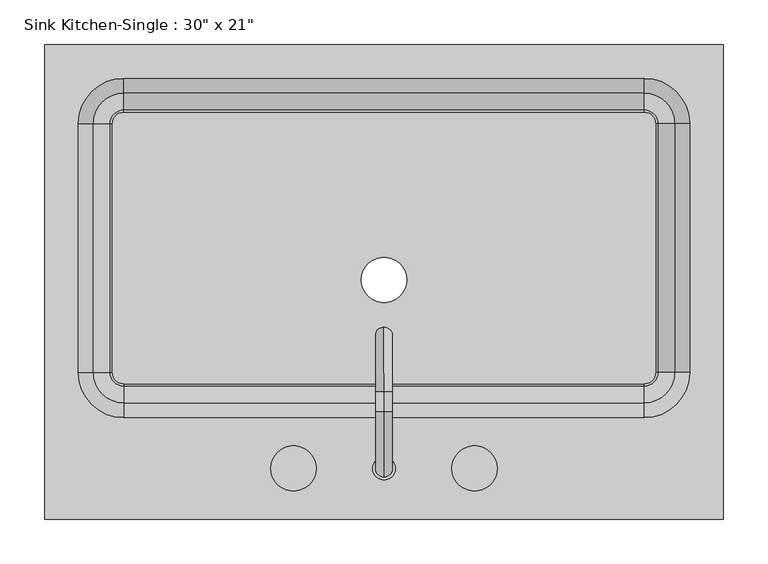
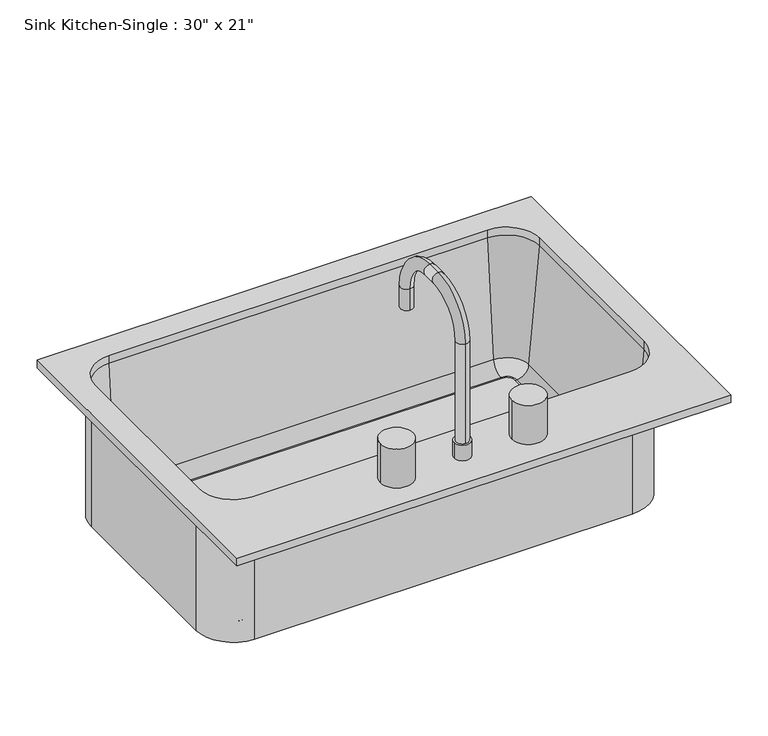
"""IFC4 building model written with IfcOpenShell, lengths in millimetres: flow terminal geometry."""

from ifc_helpers import new_model, si_unit, point, frame, frame_2d, origin, place, context, project, spatial, polyline, circle_curve, ellipse_curve, trimmed, segment, composite_curve, outline, extrude, source, transform, mapped, element, save
from ifc_brep_helpers import plane_surface, cylinder_surface, revolved_surface, advanced_brep


def flow_terminal_3ac2e542(model_context):
    return source(origin(), model_context, "Body", "SolidModel", [
        extrude(outline(composite_curve([segment(polyline([(307.7892406, -116.6454011), (-276.4107594, -116.6454011)]), True, "CONTINUOUS"), segment(trimmed(circle_curve(frame_2d((-276.4107594, -103.9454011)), 12.7), [point((-276.4107594, -116.6454011))], [point((-289.1107594, -103.9454011))], False, "CARTESIAN"), True, "CONTINUOUS"), segment(polyline([(-289.1107594, -103.9454011), (-289.1107594, 175.4545989)]), True, "CONTINUOUS"), segment(trimmed(circle_curve(frame_2d((-276.4107594, 175.4545989)), 12.7), [point((-289.1107594, 175.4545989))], [point((-276.4107594, 188.1545989))], False, "CARTESIAN"), True, "CONTINUOUS"), segment(polyline([(-276.4107594, 188.1545989), (307.7892406, 188.1545989)]), True, "CONTINUOUS"), segment(trimmed(circle_curve(frame_2d((307.7892406, 175.4545989)), 12.7), [point((307.7892406, 188.1545989))], [point((320.4892406, 175.4545989))], False, "CARTESIAN"), True, "CONTINUOUS"), segment(polyline([(320.4892406, 175.4545989), (320.4892406, -103.9454011)]), True, "CONTINUOUS"), segment(trimmed(circle_curve(frame_2d((307.7892406, -103.9454011)), 12.7), [point((320.4892406, -103.9454011))], [point((307.7892406, -116.6454011))], False, "CARTESIAN"), True, "CONTINUOUS")], self_intersect=False), holes=[composite_curve([segment(trimmed(circle_curve(frame_2d((15.6892406, 0.0)), 25.4), [point((-9.7107594, 0.0))], [point((41.0892406, 0.0))], True, "CARTESIAN"), True, "CONTINUOUS"), segment(trimmed(circle_curve(frame_2d((15.6892406, 0.0)), 25.4), [point((41.0892406, 0.0))], [point((-9.7107594, 0.0))], True, "CARTESIAN"), True, "CONTINUOUS")], self_intersect=False)]), frame((0.0, 0.0, 698.5), z_axis=(0.0, 0.0, 1.0), x_axis=(1.0, 0.0, 0.0)), (0.0, 0.0, 1.0), 9.525),
        extrude(outline(composite_curve([segment(trimmed(circle_curve(frame_2d((-85.9107594, -211.8954011)), 25.4), [point((-111.3107594, -211.8954011))], [point((-60.5107594, -211.8954011))], False, "CARTESIAN"), True, "CONTINUOUS"), segment(trimmed(circle_curve(frame_2d((-85.9107594, -211.8954011)), 25.4), [point((-60.5107594, -211.8954011))], [point((-111.3107594, -211.8954011))], False, "CARTESIAN"), True, "CONTINUOUS")], self_intersect=False)), frame((0.0, 0.0, 927.1), z_axis=(0.0, 0.0, 1.0), x_axis=(1.0, 0.0, 0.0)), (0.0, 0.0, 1.0), 63.5),
        extrude(outline(composite_curve([segment(trimmed(circle_curve(frame_2d((117.2892406, -211.8954011)), 25.4), [point((91.8892406, -211.8954011))], [point((142.6892406, -211.8954011))], False, "CARTESIAN"), True, "CONTINUOUS"), segment(trimmed(circle_curve(frame_2d((117.2892406, -211.8954011)), 25.4), [point((142.6892406, -211.8954011))], [point((91.8892406, -211.8954011))], False, "CARTESIAN"), True, "CONTINUOUS")], self_intersect=False)), frame((0.0, 0.0, 927.1), z_axis=(0.0, 0.0, 1.0), x_axis=(1.0, 0.0, 0.0)), (0.0, 0.0, 1.0), 63.5),
        advanced_brep(
        [(2.9892406, -211.8954011, 927.1), (28.3892406, -211.8954011, 927.1), (15.6892406, -221.4204011, 1114.425), (15.6892406, -221.4204011, 952.5), (15.6892406, -202.3704011, 952.5), (15.6892406, -202.3704011, 1114.425), (15.6892406, -148.3954011, 1168.4), (15.6892406, -148.3954011, 1187.45), (15.6892406, -126.1704011, 1168.4), (15.6892406, -126.1704011, 1187.45), (15.6892406, -72.1954011, 1114.425), (15.6892406, -53.1454011, 1114.425), (15.6892406, -53.1454011, 1079.5), (15.6892406, -72.1954011, 1079.5), (2.9892406, -211.8954011, 952.5), (28.3892406, -211.8954011, 952.5)],
        [
            (0, 1, circle_curve(frame((15.6892406, -211.8954011, 927.1), z_axis=(0.0, 0.0, -1.0), x_axis=(1.0, 0.0, 0.0)), 12.7)),
            (1, 0, circle_curve(frame((15.6892406, -211.8954011, 927.1), z_axis=(0.0, 0.0, -1.0), x_axis=(1.0, 0.0, 0.0)), 12.7)),
            (2, 3),
            (3, 4, circle_curve(frame((15.6892406, -211.8954011, 952.5), z_axis=(0.0, 0.0, 1.0), x_axis=(0.0, 1.0, 0.0)), 9.525)),
            (4, 5),
            (5, 2, circle_curve(frame((15.6892406, -211.8954011, 1114.425), z_axis=(0.0, 0.0, -1.0), x_axis=(0.0, 1.0, 0.0)), 9.525)),
            (4, 3, circle_curve(frame((15.6892406, -211.8954011, 952.5), z_axis=(0.0, 0.0, 1.0), x_axis=(0.0, 1.0, 0.0)), 9.525)),
            (2, 5, circle_curve(frame((15.6892406, -211.8954011, 1114.425), z_axis=(0.0, 0.0, -1.0), x_axis=(0.0, 1.0, 0.0)), 9.525)),
            (5, 6, circle_curve(frame((15.6892406, -148.3954011, 1114.425), z_axis=(-1.0, 0.0, 0.0), x_axis=(0.0, -1.0, 0.0)), 53.975)),
            (6, 7, circle_curve(frame((15.6892406, -148.3954011, 1177.925), z_axis=(0.0, -1.0, 0.0), x_axis=(0.0, 0.0, -1.0)), 9.525)),
            (7, 2, circle_curve(frame((15.6892406, -148.3954011, 1114.425), z_axis=(1.0, 0.0, 0.0), x_axis=(0.0, -1.0, 0.0)), 73.025)),
            (7, 6, circle_curve(frame((15.6892406, -148.3954011, 1177.925), z_axis=(0.0, -1.0, 0.0), x_axis=(0.0, 0.0, -1.0)), 9.525)),
            (6, 8),
            (8, 9, circle_curve(frame((15.6892406, -126.1704011, 1177.925), z_axis=(0.0, -1.0, 0.0), x_axis=(0.0, 0.0, -1.0)), 9.525)),
            (9, 7),
            (9, 8, circle_curve(frame((15.6892406, -126.1704011, 1177.925), z_axis=(0.0, -1.0, 0.0), x_axis=(0.0, 0.0, -1.0)), 9.525)),
            (8, 10, circle_curve(frame((15.6892406, -126.1704011, 1114.425), z_axis=(-1.0, 0.0, 0.0), x_axis=(0.0, 0.0, 1.0)), 53.975)),
            (10, 11, circle_curve(frame((15.6892406, -62.6704011, 1114.425), z_axis=(0.0, 0.0, 1.0), x_axis=(0.0, -1.0, 0.0)), 9.525)),
            (11, 9, circle_curve(frame((15.6892406, -126.1704011, 1114.425), z_axis=(1.0, 0.0, 0.0), x_axis=(0.0, 0.0, 1.0)), 73.025)),
            (11, 10, circle_curve(frame((15.6892406, -62.6704011, 1114.425), z_axis=(0.0, 0.0, 1.0), x_axis=(0.0, -1.0, 0.0)), 9.525)),
            (12, 13, circle_curve(frame((15.6892406, -62.6704011, 1079.5), z_axis=(0.0, 0.0, -1.0), x_axis=(0.0, -1.0, 0.0)), 9.525)),
            (13, 12, circle_curve(frame((15.6892406, -62.6704011, 1079.5), z_axis=(0.0, 0.0, -1.0), x_axis=(0.0, -1.0, 0.0)), 9.525)),
            (10, 13),
            (12, 11),
            (14, 15, circle_curve(frame((15.6892406, -211.8954011, 952.5), z_axis=(0.0, 0.0, 1.0), x_axis=(1.0, 0.0, 0.0)), 12.7)),
            (15, 14, circle_curve(frame((15.6892406, -211.8954011, 952.5), z_axis=(0.0, 0.0, 1.0), x_axis=(1.0, 0.0, 0.0)), 12.7)),
            (15, 1),
            (0, 14),
        ],
        [
            plane_surface(frame((15.6892406, -202.3704011, 927.1), z_axis=(0.0, 0.0, -1.0), x_axis=(1.0, 0.0, 0.0))),
            cylinder_surface(frame((15.6892406, -211.8954011, 927.1), z_axis=(0.0, 0.0, -1.0), x_axis=(0.0, 1.0, 0.0)), 9.525),
            revolved_surface(trimmed(ellipse_curve(frame((15.6892406, -211.8954011, 1114.425), z_axis=(0.0, 0.0, 1.0), x_axis=(0.0, 1.0, 0.0)), 9.525, 9.525), [point((15.6892406, -221.4204011, 1114.425))], [point((15.6892406, -202.3704011, 1114.425))], True, "CARTESIAN"), (15.6892406, -148.3954011, 1114.425), (1.0, 0.0, 0.0)),
            revolved_surface(trimmed(ellipse_curve(frame((15.6892406, -211.8954011, 1114.425), z_axis=(0.0, 0.0, 1.0), x_axis=(0.0, 1.0, 0.0)), 9.525, 9.525), [point((15.6892406, -202.3704011, 1114.425))], [point((15.6892406, -221.4204011, 1114.425))], True, "CARTESIAN"), (15.6892406, -148.3954011, 1114.425), (1.0, 0.0, 0.0)),
            cylinder_surface(frame((15.6892406, -148.3954011, 1177.925), z_axis=(0.0, -1.0, 0.0), x_axis=(0.0, 0.0, -1.0)), 9.525),
            revolved_surface(trimmed(ellipse_curve(frame((15.6892406, -126.1704011, 1177.925), z_axis=(0.0, 1.0, 0.0), x_axis=(0.0, 0.0, -1.0)), 9.525, 9.525), [point((15.6892406, -126.1704011, 1187.45))], [point((15.6892406, -126.1704011, 1168.4))], True, "CARTESIAN"), (15.6892406, -126.1704011, 1114.425), (1.0, 0.0, 0.0)),
            revolved_surface(trimmed(ellipse_curve(frame((15.6892406, -126.1704011, 1177.925), z_axis=(0.0, 1.0, 0.0), x_axis=(0.0, 0.0, -1.0)), 9.525, 9.525), [point((15.6892406, -126.1704011, 1168.4))], [point((15.6892406, -126.1704011, 1187.45))], True, "CARTESIAN"), (15.6892406, -126.1704011, 1114.425), (1.0, 0.0, 0.0)),
            plane_surface(frame((15.6892406, -53.1454011, 1079.5), z_axis=(0.0, 0.0, -1.0), x_axis=(-1.0, 0.0, 0.0))),
            cylinder_surface(frame((15.6892406, -62.6704011, 1114.425), z_axis=(0.0, 0.0, 1.0), x_axis=(0.0, -1.0, 0.0)), 9.525),
            plane_surface(frame((28.3892406, -211.8954011, 952.5), z_axis=(0.0, 0.0, 1.0), x_axis=(0.0, -1.0, 0.0))),
            cylinder_surface(frame((15.6892406, -211.8954011, 927.1), z_axis=(0.0, 0.0, 1.0), x_axis=(1.0, 0.0, 0.0)), 12.7),
        ],
        [
            (0, [[1, 2]]),
            (1, [[3, 4, 5, 6]]),
            (1, [[-5, 7, -3, 8]]),
            (2, [[9, 10, 11, -6]]),
            (3, [[-11, 12, -9, -8]]),
            (4, [[13, 14, 15, -10]]),
            (4, [[-15, 16, -13, -12]]),
            (5, [[17, 18, 19, -14]]),
            (6, [[-19, 20, -17, -16]]),
            (7, [[21, 22]]),
            (8, [[23, -21, 24, -18]]),
            (8, [[-24, -22, -23, -20]]),
            (9, [[25, 26], [-7, -4]]),
            (10, [[27, -1, 28, -26]]),
            (10, [[-28, -2, -27, -25]]),
        ],
    ),
        advanced_brep(
        [(396.6892406, -269.0454011, 927.1), (396.6892406, 264.3545989, 927.1), (-365.3107594, 264.3545989, 927.1), (-365.3107594, -269.0454011, 927.1), (307.7892406, -154.7454011, 927.1), (-276.4107594, -154.7454011, 927.1), (-327.2107594, -103.9454011, 927.1), (-327.2107594, 175.4545989, 927.1), (-276.4107594, 226.2545989, 927.1), (307.7892406, 226.2545989, 927.1), (358.5892406, 175.4545989, 927.1), (358.5892406, -103.9454011, 927.1), (396.6892406, -269.0454011, 914.4), (-365.3107594, -269.0454011, 914.4), (-365.3107594, 264.3545989, 914.4), (396.6892406, 264.3545989, 914.4), (364.9392406, -103.9454011, 914.4), (364.9392406, 175.4545989, 914.4), (307.7892406, 232.6045989, 914.4), (-276.4107594, 232.6045989, 914.4), (-333.5607594, 175.4545989, 914.4), (-333.5607594, -103.9454011, 914.4), (-276.4107594, -161.0954011, 914.4), (307.7892406, -161.0954011, 914.4), (358.5892406, -103.9454011, 914.4), (307.7892406, -154.7454011, 914.4), (358.5892406, 175.4545989, 914.4), (307.7892406, 226.2545989, 914.4), (-276.4107594, 226.2545989, 914.4), (-327.2107594, 175.4545989, 914.4), (-327.2107594, -103.9454011, 914.4), (-276.4107594, -154.7454011, 914.4), (364.9392406, -103.9454011, 698.5), (307.7892406, -161.0954011, 698.5), (307.7892406, -116.6454011, 698.5), (320.4892406, -103.9454011, 698.5), (307.7892406, -116.6454011, 708.025), (320.4892406, -103.9454011, 708.025), (307.7892406, -119.2338193, 708.025), (323.0776588, -103.9454011, 708.025), (307.7892406, -138.2113283, 725.4146831), (342.0551678, -103.9454011, 725.4146831), (364.9392406, 175.4545989, 698.5), (320.4892406, 175.4545989, 698.5), (320.4892406, 175.4545989, 708.025), (323.0776588, 175.4545989, 708.025), (342.0551678, 175.4545989, 725.4146831), (307.7892406, 232.6045989, 698.5), (307.7892406, 188.1545989, 698.5), (307.7892406, 188.1545989, 708.025), (307.7892406, 190.7430171, 708.025), (307.7892406, 209.7205261, 725.4146831), (-276.4107594, 232.6045989, 698.5), (-276.4107594, 188.1545989, 698.5), (-276.4107594, 188.1545989, 708.025), (-276.4107594, 190.7430171, 708.025), (-276.4107594, 209.7205261, 725.4146831), (-333.5607594, 175.4545989, 698.5), (-289.1107594, 175.4545989, 698.5), (-289.1107594, 175.4545989, 708.025), (-291.6991776, 175.4545989, 708.025), (-310.6766866, 175.4545989, 725.4146831), (-333.5607594, -103.9454011, 698.5), (-289.1107594, -103.9454011, 698.5), (-289.1107594, -103.9454011, 708.025), (-291.6991776, -103.9454011, 708.025), (-310.6766866, -103.9454011, 725.4146831), (-276.4107594, -161.0954011, 698.5), (-276.4107594, -116.6454011, 698.5), (-276.4107594, -116.6454011, 708.025), (-276.4107594, -119.2338193, 708.025), (-276.4107594, -138.2113283, 725.4146831)],
        [
            (0, 1),
            (1, 2),
            (2, 3),
            (3, 0),
            (4, 5),
            (5, 6, circle_curve(frame((-276.4107594, -103.9454011, 927.1), z_axis=(0.0, 0.0, -1.0), x_axis=(1.0, 0.0, 0.0)), 50.8)),
            (6, 7),
            (7, 8, circle_curve(frame((-276.4107594, 175.4545989, 927.1), z_axis=(0.0, 0.0, -1.0), x_axis=(1.0, 0.0, 0.0)), 50.8)),
            (8, 9),
            (9, 10, circle_curve(frame((307.7892406, 175.4545989, 927.1), z_axis=(0.0, 0.0, -1.0), x_axis=(1.0, 0.0, 0.0)), 50.8)),
            (10, 11),
            (11, 4, circle_curve(frame((307.7892406, -103.9454011, 927.1), z_axis=(0.0, 0.0, -1.0), x_axis=(1.0, 0.0, 0.0)), 50.8)),
            (12, 13),
            (13, 14),
            (14, 15),
            (15, 12),
            (16, 17),
            (17, 18, circle_curve(frame((307.7892406, 175.4545989, 914.4), z_axis=(0.0, 0.0, 1.0), x_axis=(1.0, 0.0, 0.0)), 57.15)),
            (18, 19),
            (19, 20, circle_curve(frame((-276.4107594, 175.4545989, 914.4), z_axis=(0.0, 0.0, 1.0), x_axis=(0.0, 1.0, 0.0)), 57.15)),
            (20, 21),
            (21, 22, circle_curve(frame((-276.4107594, -103.9454011, 914.4), z_axis=(0.0, 0.0, 1.0), x_axis=(-1.0, 0.0, 0.0)), 57.15)),
            (22, 23),
            (23, 16, circle_curve(frame((307.7892406, -103.9454011, 914.4), z_axis=(0.0, 0.0, 1.0), x_axis=(0.0, -1.0, 0.0)), 57.15)),
            (3, 13),
            (12, 0),
            (2, 14),
            (1, 15),
            (11, 24),
            (24, 25, circle_curve(frame((307.7892406, -103.9454011, 914.4), z_axis=(0.0, 0.0, -1.0), x_axis=(1.0, 0.0, 0.0)), 50.8)),
            (25, 4),
            (10, 26),
            (26, 24),
            (9, 27),
            (27, 26, circle_curve(frame((307.7892406, 175.4545989, 914.4), z_axis=(0.0, 0.0, -1.0), x_axis=(1.0, 0.0, 0.0)), 50.8)),
            (8, 28),
            (28, 27),
            (7, 29),
            (29, 28, circle_curve(frame((-276.4107594, 175.4545989, 914.4), z_axis=(0.0, 0.0, -1.0), x_axis=(1.0, 0.0, 0.0)), 50.8)),
            (6, 30),
            (30, 29),
            (5, 31),
            (31, 30, circle_curve(frame((-276.4107594, -103.9454011, 914.4), z_axis=(0.0, 0.0, -1.0), x_axis=(1.0, 0.0, 0.0)), 50.8)),
            (25, 31),
            (32, 16),
            (23, 33),
            (33, 32, circle_curve(frame((307.7892406, -103.9454011, 698.5), z_axis=(0.0, 0.0, 1.0), x_axis=(0.0, -1.0, 0.0)), 57.15)),
            (33, 34),
            (34, 35, circle_curve(frame((307.7892406, -103.9454011, 698.5), z_axis=(0.0, 0.0, 1.0), x_axis=(0.0, -1.0, 0.0)), 12.7)),
            (35, 32),
            (34, 36),
            (36, 37, circle_curve(frame((307.7892406, -103.9454011, 708.025), z_axis=(0.0, 0.0, 1.0), x_axis=(0.0, -1.0, 0.0)), 12.7)),
            (37, 35),
            (36, 38),
            (38, 39, circle_curve(frame((307.7892406, -103.9454011, 708.025), z_axis=(0.0, 0.0, 1.0), x_axis=(0.0, -1.0, 0.0)), 15.2884182)),
            (39, 37),
            (38, 40, circle_curve(frame((307.7892406, -119.2338193, 727.075), z_axis=(-1.0, 0.0, 0.0), x_axis=(0.0, -1.0, 0.0)), 19.05)),
            (40, 41, circle_curve(frame((307.7892406, -103.9454011, 725.4146831), z_axis=(0.0, 0.0, 1.0), x_axis=(0.0, -1.0, 0.0)), 34.2659272)),
            (41, 39, circle_curve(frame((323.0776588, -103.9454011, 727.075), z_axis=(0.0, 1.0, 0.0), x_axis=(1.0, 0.0, 0.0)), 19.05)),
            (40, 25),
            (24, 41),
            (32, 42),
            (42, 17),
            (35, 43),
            (43, 42),
            (37, 44),
            (44, 43),
            (39, 45),
            (45, 44),
            (41, 46),
            (46, 45, circle_curve(frame((323.0776588, 175.4545989, 727.075), z_axis=(0.0, 1.0, 0.0), x_axis=(1.0, 0.0, 0.0)), 19.05)),
            (26, 46),
            (42, 47, circle_curve(frame((307.7892406, 175.4545989, 698.5), z_axis=(0.0, 0.0, 1.0), x_axis=(1.0, 0.0, 0.0)), 57.15)),
            (47, 18),
            (43, 48, circle_curve(frame((307.7892406, 175.4545989, 698.5), z_axis=(0.0, 0.0, 1.0), x_axis=(1.0, 0.0, 0.0)), 12.7)),
            (48, 47),
            (44, 49, circle_curve(frame((307.7892406, 175.4545989, 708.025), z_axis=(0.0, 0.0, 1.0), x_axis=(1.0, 0.0, 0.0)), 12.7)),
            (49, 48),
            (45, 50, circle_curve(frame((307.7892406, 175.4545989, 708.025), z_axis=(0.0, 0.0, 1.0), x_axis=(1.0, 0.0, 0.0)), 15.2884182)),
            (50, 49),
            (46, 51, circle_curve(frame((307.7892406, 175.4545989, 725.4146831), z_axis=(0.0, 0.0, 1.0), x_axis=(1.0, 0.0, 0.0)), 34.2659272)),
            (51, 50, circle_curve(frame((307.7892406, 190.7430171, 727.075), z_axis=(-1.0, 0.0, 0.0), x_axis=(0.0, 1.0, 0.0)), 19.05)),
            (27, 51),
            (47, 52),
            (52, 19),
            (48, 53),
            (53, 52),
            (49, 54),
            (54, 53),
            (50, 55),
            (55, 54),
            (51, 56),
            (56, 55, circle_curve(frame((-276.4107594, 190.7430171, 727.075), z_axis=(-1.0, 0.0, 0.0), x_axis=(0.0, 1.0, 0.0)), 19.05)),
            (28, 56),
            (52, 57, circle_curve(frame((-276.4107594, 175.4545989, 698.5), z_axis=(0.0, 0.0, 1.0), x_axis=(0.0, 1.0, 0.0)), 57.15)),
            (57, 20),
            (53, 58, circle_curve(frame((-276.4107594, 175.4545989, 698.5), z_axis=(0.0, 0.0, 1.0), x_axis=(0.0, 1.0, 0.0)), 12.7)),
            (58, 57),
            (54, 59, circle_curve(frame((-276.4107594, 175.4545989, 708.025), z_axis=(0.0, 0.0, 1.0), x_axis=(0.0, 1.0, 0.0)), 12.7)),
            (59, 58),
            (55, 60, circle_curve(frame((-276.4107594, 175.4545989, 708.025), z_axis=(0.0, 0.0, 1.0), x_axis=(0.0, 1.0, 0.0)), 15.2884182)),
            (60, 59),
            (56, 61, circle_curve(frame((-276.4107594, 175.4545989, 725.4146831), z_axis=(0.0, 0.0, 1.0), x_axis=(0.0, 1.0, 0.0)), 34.2659272)),
            (61, 60, circle_curve(frame((-291.6991776, 175.4545989, 727.075), z_axis=(0.0, -1.0, 0.0), x_axis=(-1.0, 0.0, 0.0)), 19.05)),
            (29, 61),
            (57, 62),
            (62, 21),
            (58, 63),
            (63, 62),
            (59, 64),
            (64, 63),
            (60, 65),
            (65, 64),
            (61, 66),
            (66, 65, circle_curve(frame((-291.6991776, -103.9454011, 727.075), z_axis=(0.0, -1.0, 0.0), x_axis=(-1.0, 0.0, 0.0)), 19.05)),
            (30, 66),
            (62, 67, circle_curve(frame((-276.4107594, -103.9454011, 698.5), z_axis=(0.0, 0.0, 1.0), x_axis=(-1.0, 0.0, 0.0)), 57.15)),
            (67, 22),
            (63, 68, circle_curve(frame((-276.4107594, -103.9454011, 698.5), z_axis=(0.0, 0.0, 1.0), x_axis=(-1.0, 0.0, 0.0)), 12.7)),
            (68, 67),
            (64, 69, circle_curve(frame((-276.4107594, -103.9454011, 708.025), z_axis=(0.0, 0.0, 1.0), x_axis=(-1.0, 0.0, 0.0)), 12.7)),
            (69, 68),
            (65, 70, circle_curve(frame((-276.4107594, -103.9454011, 708.025), z_axis=(0.0, 0.0, 1.0), x_axis=(-1.0, 0.0, 0.0)), 15.2884182)),
            (70, 69),
            (66, 71, circle_curve(frame((-276.4107594, -103.9454011, 725.4146831), z_axis=(0.0, 0.0, 1.0), x_axis=(-1.0, 0.0, 0.0)), 34.2659272)),
            (71, 70, circle_curve(frame((-276.4107594, -119.2338193, 727.075), z_axis=(1.0, 0.0, 0.0), x_axis=(0.0, -1.0, 0.0)), 19.05)),
            (31, 71),
            (67, 33),
            (68, 34),
            (69, 36),
            (70, 38),
            (71, 40),
        ],
        [
            plane_surface(frame((-365.3107594, -269.0454011, 927.1), z_axis=(0.0, 0.0, 1.0), x_axis=(-1.0, 0.0, 0.0))),
            plane_surface(frame((-365.3107594, -269.0454011, 914.4), z_axis=(0.0, 0.0, -1.0), x_axis=(1.0, 0.0, 0.0))),
            plane_surface(frame((396.6892406, -269.0454011, 927.1), z_axis=(0.0, -1.0, 0.0), x_axis=(0.0, 0.0, -1.0))),
            plane_surface(frame((-365.3107594, -269.0454011, 927.1), z_axis=(-1.0, 0.0, 0.0), x_axis=(0.0, 0.0, -1.0))),
            plane_surface(frame((-365.3107594, 264.3545989, 927.1), z_axis=(0.0, 1.0, 0.0), x_axis=(0.0, 0.0, -1.0))),
            plane_surface(frame((396.6892406, 264.3545989, 927.1), z_axis=(1.0, 0.0, 0.0), x_axis=(0.0, 0.0, -1.0))),
            revolved_surface(polyline([(358.58924060000004, -103.9454011, 914.4), (358.58924060000004, -103.9454011, 927.1)]), (307.7892406, -103.9454011, 0.0), (0.0, 0.0, -1.0)),
            plane_surface(frame((358.5892406, -103.9454011, 927.1), z_axis=(-1.0, 0.0, 0.0), x_axis=(0.0, 0.0, -1.0))),
            revolved_surface(polyline([(358.58924060000004, 175.4545989, 914.4), (358.58924060000004, 175.4545989, 927.1)]), (307.7892406, 175.4545989, 0.0), (0.0, 0.0, -1.0)),
            plane_surface(frame((307.7892406, 226.2545989, 927.1), z_axis=(0.0, -1.0, 0.0), x_axis=(0.0, 0.0, -1.0))),
            revolved_surface(polyline([(-225.6107594, 175.4545989, 914.4), (-225.6107594, 175.4545989, 927.1)]), (-276.4107594, 175.4545989, 0.0), (0.0, 0.0, -1.0)),
            plane_surface(frame((-327.2107594, 175.4545989, 927.1), z_axis=(1.0, 0.0, 0.0), x_axis=(0.0, 0.0, -1.0))),
            revolved_surface(polyline([(-225.6107594, -103.9454011, 914.4), (-225.6107594, -103.9454011, 927.1)]), (-276.4107594, -103.9454011, 0.0), (0.0, 0.0, -1.0)),
            plane_surface(frame((-276.4107594, -154.7454011, 927.1), z_axis=(0.0, 1.0, 0.0), x_axis=(0.0, 0.0, -1.0))),
            cylinder_surface(frame((307.7892406, -103.9454011, 0.0), z_axis=(0.0, 0.0, -1.0), x_axis=(0.0, -1.0, 0.0)), 57.15),
            plane_surface(frame((307.7892406, -103.9454011, 698.5), z_axis=(0.0, 0.0, -1.0), x_axis=(0.0, -1.0, 0.0))),
            revolved_surface(polyline([(307.7892406, -116.6454011, 698.5), (307.7892406, -116.6454011, 708.025)]), (307.7892406, -103.9454011, 0.0), (0.0, 0.0, -1.0)),
            plane_surface(frame((307.7892406, -103.9454011, 708.025), z_axis=(0.0, 0.0, 1.0), x_axis=(0.0, -1.0, 0.0))),
            revolved_surface(trimmed(ellipse_curve(frame((307.7892406, -119.2338193, 727.075), z_axis=(-1.0, 0.0, 0.0), x_axis=(0.0, -1.0, 0.0)), 19.05, 19.05), [point((307.7892406, -119.2338193, 708.025))], [point((307.7892406, -138.2113283, 725.4146831))], True, "CARTESIAN"), (307.7892406, -103.9454011, 0.0), (0.0, 0.0, -1.0)),
            revolved_surface(polyline([(307.7892406, -138.2113283, 725.4146831), (307.7892406, -154.7454011, 914.4)]), (307.7892406, -103.9454011, 0.0), (0.0, 0.0, -1.0)),
            plane_surface(frame((364.9392406, -103.9454011, 914.4), z_axis=(1.0, 0.0, 0.0), x_axis=(0.0, 1.0, 0.0))),
            plane_surface(frame((364.9392406, -103.9454011, 698.5), z_axis=(0.0, 0.0, -1.0), x_axis=(0.0, 1.0, 0.0))),
            plane_surface(frame((320.4892406, -103.9454011, 698.5), z_axis=(-1.0, 0.0, 0.0), x_axis=(0.0, 1.0, 0.0))),
            plane_surface(frame((320.4892406, -103.9454011, 708.025), z_axis=(0.0, 0.0, 1.0), x_axis=(0.0, 1.0, 0.0))),
            revolved_surface(polyline([(342.1276588, 175.45459889999998, 727.075), (342.1276588, -103.9454011, 727.075)]), (323.0776588, -103.9454011, 727.075), (0.0, 1.0, 0.0)),
            plane_surface(frame((342.0551678, -103.9454011, 725.4146831), z_axis=(-0.9961946980917442, 0.0, 0.08715574274767306), x_axis=(0.0, 1.0, 0.0))),
            cylinder_surface(frame((307.7892406, 175.4545989, 0.0), z_axis=(0.0, 0.0, -1.0), x_axis=(1.0, 0.0, 0.0)), 57.15),
            plane_surface(frame((307.7892406, 175.4545989, 698.5), z_axis=(0.0, 0.0, -1.0), x_axis=(1.0, 0.0, 0.0))),
            revolved_surface(polyline([(320.4892406, 175.4545989, 698.5), (320.4892406, 175.4545989, 708.025)]), (307.7892406, 175.4545989, 0.0), (0.0, 0.0, -1.0)),
            plane_surface(frame((307.7892406, 175.4545989, 708.025), z_axis=(0.0, 0.0, 1.0), x_axis=(1.0, 0.0, 0.0))),
            revolved_surface(trimmed(ellipse_curve(frame((323.0776588, 175.4545989, 727.075), z_axis=(0.0, -1.0, 0.0), x_axis=(1.0, 0.0, 0.0)), 19.05, 19.05), [point((323.0776588, 175.4545989, 708.025))], [point((342.0551678, 175.4545989, 725.4146831))], True, "CARTESIAN"), (307.7892406, 175.4545989, 0.0), (0.0, 0.0, -1.0)),
            revolved_surface(polyline([(342.0551678, 175.4545989, 725.4146831), (358.5892406, 175.4545989, 914.4)]), (307.7892406, 175.4545989, 0.0), (0.0, 0.0, -1.0)),
            plane_surface(frame((307.7892406, 232.6045989, 914.4), z_axis=(0.0, 1.0, 0.0), x_axis=(-1.0, 0.0, 0.0))),
            plane_surface(frame((307.7892406, 232.6045989, 698.5), z_axis=(0.0, 0.0, -1.0), x_axis=(-1.0, 0.0, 0.0))),
            plane_surface(frame((307.7892406, 188.1545989, 698.5), z_axis=(0.0, -1.0, 0.0), x_axis=(-1.0, 0.0, 0.0))),
            plane_surface(frame((307.7892406, 188.1545989, 708.025), z_axis=(0.0, 0.0, 1.0), x_axis=(-1.0, 0.0, 0.0))),
            revolved_surface(polyline([(-276.4107594, 209.79301710000001, 727.075), (307.7892406, 209.79301710000001, 727.075)]), (307.7892406, 190.7430171, 727.075), (-1.0, 0.0, 0.0)),
            plane_surface(frame((307.7892406, 209.7205261, 725.4146831), z_axis=(0.0, -0.9961946980917442, 0.08715574274767306), x_axis=(-1.0, 0.0, 0.0))),
            cylinder_surface(frame((-276.4107594, 175.4545989, 0.0), z_axis=(0.0, 0.0, -1.0), x_axis=(0.0, 1.0, 0.0)), 57.15),
            plane_surface(frame((-276.4107594, 175.4545989, 698.5), z_axis=(0.0, 0.0, -1.0), x_axis=(0.0, 1.0, 0.0))),
            revolved_surface(polyline([(-276.4107594, 188.1545989, 698.5), (-276.4107594, 188.1545989, 708.025)]), (-276.4107594, 175.4545989, 0.0), (0.0, 0.0, -1.0)),
            plane_surface(frame((-276.4107594, 175.4545989, 708.025), z_axis=(0.0, 0.0, 1.0), x_axis=(0.0, 1.0, 0.0))),
            revolved_surface(trimmed(ellipse_curve(frame((-276.4107594, 190.7430171, 727.075), z_axis=(1.0, 0.0, 0.0), x_axis=(0.0, 1.0, 0.0)), 19.05, 19.05), [point((-276.4107594, 190.7430171, 708.025))], [point((-276.4107594, 209.7205261, 725.4146831))], True, "CARTESIAN"), (-276.4107594, 175.4545989, 0.0), (0.0, 0.0, -1.0)),
            revolved_surface(polyline([(-276.4107594, 209.7205261, 725.4146831), (-276.4107594, 226.2545989, 914.4)]), (-276.4107594, 175.4545989, 0.0), (0.0, 0.0, -1.0)),
            plane_surface(frame((-333.5607594, 175.4545989, 914.4), z_axis=(-1.0, 0.0, 0.0), x_axis=(0.0, -1.0, 0.0))),
            plane_surface(frame((-333.5607594, 175.4545989, 698.5), z_axis=(0.0, 0.0, -1.0), x_axis=(0.0, -1.0, 0.0))),
            plane_surface(frame((-289.1107594, 175.4545989, 698.5), z_axis=(1.0, 0.0, 0.0), x_axis=(0.0, -1.0, 0.0))),
            plane_surface(frame((-289.1107594, 175.4545989, 708.025), z_axis=(0.0, 0.0, 1.0), x_axis=(0.0, -1.0, 0.0))),
            revolved_surface(polyline([(-310.7491776, -103.94540109999997, 727.075), (-310.7491776, 175.4545989, 727.075)]), (-291.6991776, 175.4545989, 727.075), (0.0, -1.0, 0.0)),
            plane_surface(frame((-310.6766866, 175.4545989, 725.4146831), z_axis=(0.9961946980917442, 0.0, 0.08715574274767306), x_axis=(0.0, -1.0, 0.0))),
            cylinder_surface(frame((-276.4107594, -103.9454011, 0.0), z_axis=(0.0, 0.0, -1.0), x_axis=(-1.0, 0.0, 0.0)), 57.15),
            plane_surface(frame((-276.4107594, -103.9454011, 698.5), z_axis=(0.0, 0.0, -1.0), x_axis=(-1.0, 0.0, 0.0))),
            revolved_surface(polyline([(-289.1107594, -103.9454011, 698.5), (-289.1107594, -103.9454011, 708.025)]), (-276.4107594, -103.9454011, 0.0), (0.0, 0.0, -1.0)),
            plane_surface(frame((-276.4107594, -103.9454011, 708.025), z_axis=(0.0, 0.0, 1.0), x_axis=(-1.0, 0.0, 0.0))),
            revolved_surface(trimmed(ellipse_curve(frame((-291.6991776, -103.9454011, 727.075), z_axis=(0.0, 1.0, 0.0), x_axis=(-1.0, 0.0, 0.0)), 19.05, 19.05), [point((-291.6991776, -103.9454011, 708.025))], [point((-310.6766866, -103.9454011, 725.4146831))], True, "CARTESIAN"), (-276.4107594, -103.9454011, 0.0), (0.0, 0.0, -1.0)),
            revolved_surface(polyline([(-310.6766866, -103.9454011, 725.4146831), (-327.2107594, -103.9454011, 914.4)]), (-276.4107594, -103.9454011, 0.0), (0.0, 0.0, -1.0)),
            plane_surface(frame((-276.4107594, -161.0954011, 914.4), z_axis=(0.0, -1.0, 0.0), x_axis=(1.0, 0.0, 0.0))),
            plane_surface(frame((-276.4107594, -161.0954011, 698.5), z_axis=(0.0, 0.0, -1.0), x_axis=(1.0, 0.0, 0.0))),
            plane_surface(frame((-276.4107594, -116.6454011, 698.5), z_axis=(0.0, 1.0, 0.0), x_axis=(1.0, 0.0, 0.0))),
            plane_surface(frame((-276.4107594, -116.6454011, 708.025), z_axis=(0.0, 0.0, 1.0), x_axis=(1.0, 0.0, 0.0))),
            revolved_surface(polyline([(307.7892406, -138.2838193, 727.075), (-276.4107594, -138.2838193, 727.075)]), (-276.4107594, -119.2338193, 727.075), (1.0, 0.0, 0.0)),
            plane_surface(frame((-276.4107594, -138.2113283, 725.4146831), z_axis=(0.0, 0.9961946980917442, 0.08715574274767306), x_axis=(1.0, 0.0, 0.0))),
        ],
        [
            (0, [[1, 2, 3, 4], [5, 6, 7, 8, 9, 10, 11, 12]]),
            (1, [[13, 14, 15, 16], [17, 18, 19, 20, 21, 22, 23, 24]]),
            (2, [[25, -13, 26, -4]]),
            (3, [[27, -14, -25, -3]]),
            (4, [[28, -15, -27, -2]]),
            (5, [[-26, -16, -28, -1]]),
            (6, [[29, 30, 31, -12]]),
            (7, [[32, 33, -29, -11]]),
            (8, [[34, 35, -32, -10]]),
            (9, [[36, 37, -34, -9]]),
            (10, [[38, 39, -36, -8]]),
            (11, [[40, 41, -38, -7]]),
            (12, [[42, 43, -40, -6]]),
            (13, [[-31, 44, -42, -5]]),
            (14, [[45, -24, 46, 47]]),
            (15, [[48, 49, 50, -47]]),
            (16, [[51, 52, 53, -49]]),
            (17, [[54, 55, 56, -52]]),
            (18, [[57, 58, 59, -55]]),
            (19, [[60, -30, 61, -58]]),
            (20, [[62, 63, -17, -45]]),
            (21, [[64, 65, -62, -50]]),
            (22, [[66, 67, -64, -53]]),
            (23, [[68, 69, -66, -56]]),
            (24, [[70, 71, -68, -59]]),
            (25, [[-33, 72, -70, -61]]),
            (26, [[73, 74, -18, -63]]),
            (27, [[75, 76, -73, -65]]),
            (28, [[77, 78, -75, -67]]),
            (29, [[79, 80, -77, -69]]),
            (30, [[81, 82, -79, -71]]),
            (31, [[-35, 83, -81, -72]]),
            (32, [[84, 85, -19, -74]]),
            (33, [[86, 87, -84, -76]]),
            (34, [[88, 89, -86, -78]]),
            (35, [[90, 91, -88, -80]]),
            (36, [[92, 93, -90, -82]]),
            (37, [[-37, 94, -92, -83]]),
            (38, [[95, 96, -20, -85]]),
            (39, [[97, 98, -95, -87]]),
            (40, [[99, 100, -97, -89]]),
            (41, [[101, 102, -99, -91]]),
            (42, [[103, 104, -101, -93]]),
            (43, [[-39, 105, -103, -94]]),
            (44, [[106, 107, -21, -96]]),
            (45, [[108, 109, -106, -98]]),
            (46, [[110, 111, -108, -100]]),
            (47, [[112, 113, -110, -102]]),
            (48, [[114, 115, -112, -104]]),
            (49, [[-41, 116, -114, -105]]),
            (50, [[117, 118, -22, -107]]),
            (51, [[119, 120, -117, -109]]),
            (52, [[121, 122, -119, -111]]),
            (53, [[123, 124, -121, -113]]),
            (54, [[125, 126, -123, -115]]),
            (55, [[-43, 127, -125, -116]]),
            (56, [[-23, -118, 128, -46]]),
            (57, [[-128, -120, 129, -48]]),
            (58, [[-129, -122, 130, -51]]),
            (59, [[-130, -124, 131, -54]]),
            (60, [[-131, -126, 132, -57]]),
            (61, [[-132, -127, -44, -60]]),
        ],
    ),
    ])


if __name__ == "__main__":
    model = new_model("IFC4")
    model_context = context("Model", 3, world=origin())
    ifc_project = project(units=[si_unit("LENGTHUNIT", "METRE", prefix="MILLI")], contexts=[model_context])
    site = spatial("IfcSite", under=ifc_project)
    building = spatial("IfcBuilding", under=site)
    placement = place(None, origin())
    flow_terminal_shape = flow_terminal_3ac2e542(model_context)
    element("IfcFlowTerminal", 1, ObjectType="Sink Kitchen-Single : 30\" x 21\"", at=placement, inside=building, context=model_context, shape_type="MappedRepresentation", body=[
        mapped(flow_terminal_shape, transform((0.0, 0.0, 0.0), x_axis=(1.0, 0.0, 0.0), y_axis=(0.0, 1.0, 0.0), z_axis=(0.0, 0.0, 1.0))),
    ])
    save(model, "model.ifc")

# Revit data of these elements
# Type "Sink Kitchen-Single : 30\" x 21\""
#   Assembly Code = "D2010410"
#   Counter Height = 3' - 0"
#   Depth = 1' - 9"
#   Width = 2' - 6"
#   Faucet Material = Steel, Polished
#   Sink Material = Steel, Polished
#   Default Elevation = 0
# Element 1 (IfcFlowTerminal, "Sink Kitchen-Single : 30\" x 21\"")
#   Materials on its faces: "Steel, Polished"
# Materials
#   "Steel, Polished": class "Metal", colour RGB 192 192 192, transparency 0, Description = "Polished steel", Cost = 0
